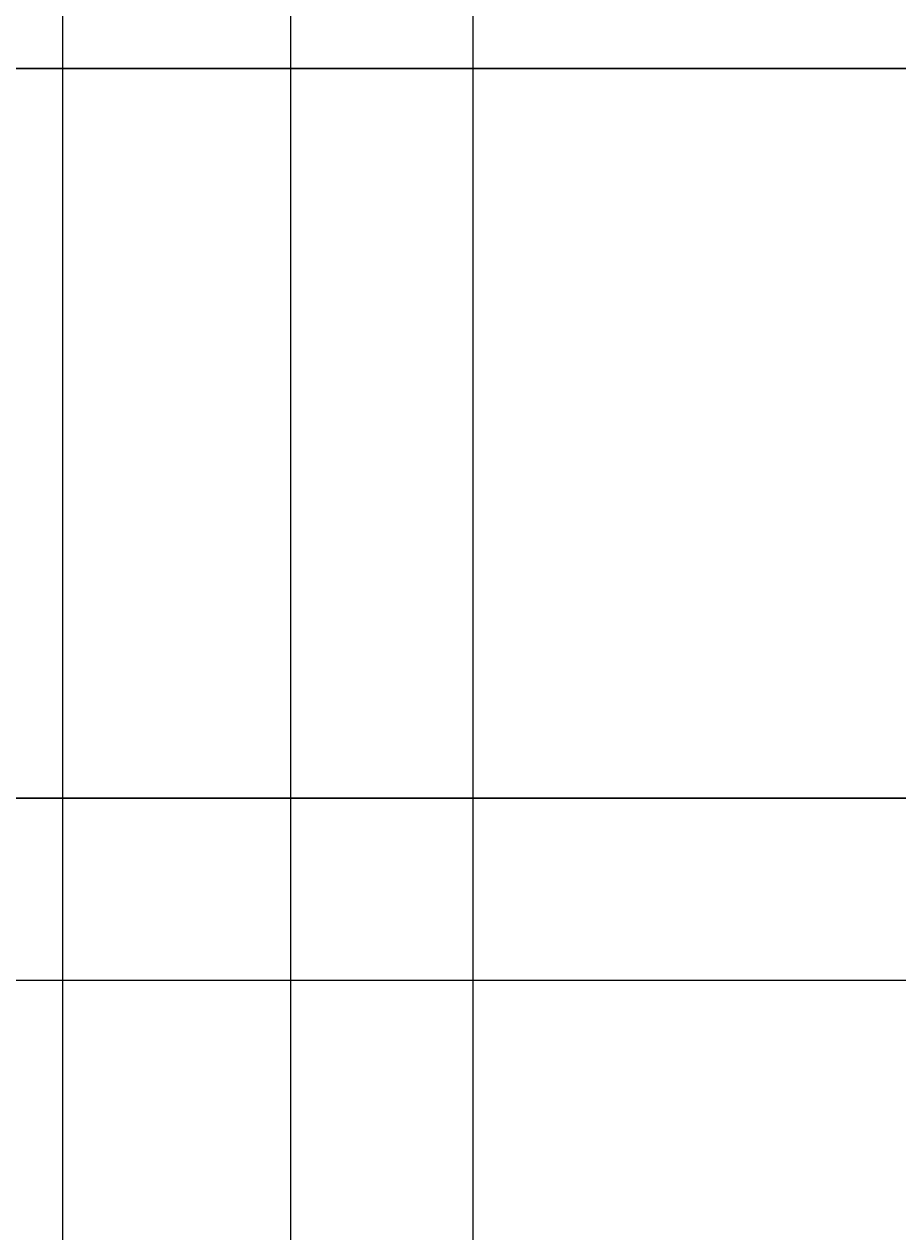
# Model space of a CAD drawing. Units: feet. Extents: x 105 to 1094, y -88 to 588.
# Tile 32 of 59: x 365 to 384, y 518 to 544. Entities that reach past the tile are written whole.
import ezdxf

# ---------------------------------------------------------------- set-up
doc = ezdxf.new("R2010")
doc.units = ezdxf.units.FT
doc.header["$MEASUREMENT"] = 0
doc.layers.add('A-ANNO-DIMS', color=2, linetype='Continuous', lineweight=18)
doc.layers.add('A-FLOR-PROJ', color=8, linetype='Continuous', lineweight=25)
doc.styles.get("Standard").update_dxf_attribs({"font": 'arial.ttf'})
doc.dimstyles.get("Standard").update_dxf_attribs({"dimtxt": 0.18, "dimasz": 0.18, "dimexe": 0.18, "dimexo": 0.0625, "dimgap": 0.09, "dimtad": 0, "dimtih": 1, "dimtoh": 1, "dimdec": 4, "dimzin": 0, "dimdsep": 46, "dimtxsty": 'Standard', "dimcen": 0.09, "dimadec": 0, "dimazin": 0, "dimtfac": 1, "dimtdec": 4, "dimtofl": 0, "dimtmove": 0, "dimatfit": 3, "dimfxl": 1, "dimtolj": 1, "dimtzin": 0, "dimarcsym": 0})

# ---------------------------------------------------------------- blocks, each defined once
blk = doc.blocks.new('*D21')
at = {"layer": 'A-ANNO-DIMS', "color": 0, "lineweight": -2, "transparency": 16777216}
for p, q in [((849.626, 543.081), (105.458, 543.081)), ((105.638, 542.901), (105.638, 250.263)), ((105.638, -42.739), (105.638, 249.899)), ((849.626, -42.919), (105.458, -42.919))]:
    blk.add_line(p, q, dxfattribs=at)
at = {"layer": 'A-ANNO-DIMS', "color": 0, "transparency": 16777216}
for points in [[(105.608, 542.901), (105.668, 542.901), (105.638, 543.081)], [(105.608, -42.739), (105.668, -42.739), (105.638, -42.919)]]:
    blk.add_solid(points, dxfattribs=at)
at = {"layer": 'Defpoints', "color": 0, "transparency": 16777216}
for p in [(105.638, 543.081), (849.688, 543.081), (849.688, -42.919)]:
    blk.add_point(p, dxfattribs=at)
at = {"layer": 'A-ANNO-DIMS', "color": 0, "transparency": 16777216, "insert": (105.638, 250.081), "char_height": 0.18, "attachment_point": 5}
blk.add_mtext('\\A1;586', dxfattribs=at)
blk = doc.blocks.new('*D24')
at = {"layer": 'A-ANNO-DIMS', "color": 0, "lineweight": -2, "transparency": 16777216}
for p, q in [((349.688, 543.144), (349.688, 588.311)), ((438.688, 527.144), (438.688, 588.311)), ((349.868, 588.131), (393.969, 588.131)), ((438.508, 588.131), (394.408, 588.131))]:
    blk.add_line(p, q, dxfattribs=at)
at = {"layer": 'A-ANNO-DIMS', "color": 0, "transparency": 16777216}
for points in [[(349.868, 588.161), (349.868, 588.101), (349.688, 588.131)], [(438.508, 588.161), (438.508, 588.101), (438.688, 588.131)]]:
    blk.add_solid(points, dxfattribs=at)
at = {"layer": 'Defpoints', "color": 0, "transparency": 16777216}
for p in [(438.688, 588.131), (349.688, 543.081), (438.688, 527.081)]:
    blk.add_point(p, dxfattribs=at)
at = {"layer": 'A-ANNO-DIMS', "color": 0, "transparency": 16777216, "insert": (394.188, 588.131), "char_height": 0.18, "attachment_point": 5}
blk.add_mtext('\\A1;89', dxfattribs=at)
blk = doc.blocks.new('*D30')
at = {"layer": 'A-ANNO-DIMS', "color": 0, "lineweight": -2, "transparency": 16777216}
for p, q in [((349.751, 543.081), (1093.918, 543.081)), ((1093.738, 542.901), (1093.738, 535.263)), ((1093.738, 527.261), (1093.738, 534.899)), ((349.751, 527.081), (1093.918, 527.081))]:
    blk.add_line(p, q, dxfattribs=at)
at = {"layer": 'A-ANNO-DIMS', "color": 0, "transparency": 16777216}
for points in [[(1093.708, 542.901), (1093.768, 542.901), (1093.738, 543.081)], [(1093.708, 527.261), (1093.768, 527.261), (1093.738, 527.081)]]:
    blk.add_solid(points, dxfattribs=at)
at = {"layer": 'Defpoints', "color": 0, "transparency": 16777216}
for p in [(349.688, 543.081), (349.688, 527.081), (1093.738, 527.081)]:
    blk.add_point(p, dxfattribs=at)
at = {"layer": 'A-ANNO-DIMS', "color": 0, "transparency": 16777216, "insert": (1093.738, 535.081), "char_height": 0.18, "attachment_point": 5}
blk.add_mtext('\\A1;16', dxfattribs=at)
blk = doc.blocks.new('*D39')
at = {"layer": 'A-ANNO-DIMS', "color": 0, "lineweight": -2, "transparency": 16777216}
for p, q in [((294.688, 204.144), (294.688, 588.311)), ((370.688, 204.144), (370.688, 588.311)), ((294.868, 588.131), (332.47, 588.131)), ((370.508, 588.131), (332.906, 588.131))]:
    blk.add_line(p, q, dxfattribs=at)
at = {"layer": 'A-ANNO-DIMS', "color": 0, "transparency": 16777216}
for points in [[(294.868, 588.161), (294.868, 588.101), (294.688, 588.131)], [(370.508, 588.161), (370.508, 588.101), (370.688, 588.131)]]:
    blk.add_solid(points, dxfattribs=at)
at = {"layer": 'Defpoints', "color": 0, "transparency": 16777216}
for p in [(370.688, 588.131), (294.688, 204.081), (370.688, 204.081)]:
    blk.add_point(p, dxfattribs=at)
at = {"layer": 'A-ANNO-DIMS', "color": 0, "transparency": 16777216, "insert": (332.688, 588.131), "char_height": 0.18, "attachment_point": 5}
blk.add_mtext('\\A1;76', dxfattribs=at)
blk = doc.blocks.new('*D53')
at = {"layer": 'A-ANNO-DIMS', "color": 0, "lineweight": -2, "transparency": 16777216}
for p, q in [((365.688, 394.144), (365.688, 588.311)), ((414.688, 394.144), (414.688, 588.311)), ((365.868, 588.131), (389.966, 588.131)), ((414.508, 588.131), (390.411, 588.131))]:
    blk.add_line(p, q, dxfattribs=at)
at = {"layer": 'A-ANNO-DIMS', "color": 0, "transparency": 16777216}
for points in [[(365.868, 588.161), (365.868, 588.101), (365.688, 588.131)], [(414.508, 588.161), (414.508, 588.101), (414.688, 588.131)]]:
    blk.add_solid(points, dxfattribs=at)
at = {"layer": 'Defpoints', "color": 0, "transparency": 16777216}
for p in [(365.688, 588.131), (365.688, 394.081), (414.688, 394.081)]:
    blk.add_point(p, dxfattribs=at)
at = {"layer": 'A-ANNO-DIMS', "color": 0, "transparency": 16777216, "insert": (390.188, 588.131), "char_height": 0.18, "attachment_point": 5}
blk.add_mtext('\\A1;49', dxfattribs=at)
blk = doc.blocks.new('*D56')
at = {"layer": 'A-ANNO-DIMS', "color": 0, "lineweight": -2, "transparency": 16777216}
for p, q in [((374.688, 252.144), (374.688, 588.311)), ((422.688, 252.144), (422.688, 588.311)), ((374.868, 588.131), (398.466, 588.131)), ((422.508, 588.131), (398.911, 588.131))]:
    blk.add_line(p, q, dxfattribs=at)
at = {"layer": 'A-ANNO-DIMS', "color": 0, "transparency": 16777216}
for points in [[(374.868, 588.161), (374.868, 588.101), (374.688, 588.131)], [(422.508, 588.161), (422.508, 588.101), (422.688, 588.131)]]:
    blk.add_solid(points, dxfattribs=at)
at = {"layer": 'Defpoints', "color": 0, "transparency": 16777216}
for p in [(422.688, 588.131), (374.688, 252.081), (422.688, 252.081)]:
    blk.add_point(p, dxfattribs=at)
at = {"layer": 'A-ANNO-DIMS', "color": 0, "transparency": 16777216, "insert": (398.688, 588.131), "char_height": 0.18, "attachment_point": 5}
blk.add_mtext('\\A1;48', dxfattribs=at)

msp = doc.modelspace()

# ---------------------------------------------------------------- linework, layer by layer
at = {"layer": 'A-FLOR-PROJ'}
for p, q in [((438.6883, 527.0812), (349.6883, 527.0812)), ((434.6883, 523.0812), (349.6883, 523.0812))]:
    msp.add_line(p, q, dxfattribs=at)

# ---------------------------------------------------------------- dimensions: what is measured, and where the dimension line sits
at = {"layer": 'A-ANNO-DIMS'}
for base, p1, p2, picture, middle in [((370.6883, 588.1312), (294.6883, 204.0812), (370.6883, 204.0812), '*D39', (332.6883, 588.1312)), ((438.6883, 588.1312), (349.6883, 543.0812), (438.6883, 527.0812), '*D24', (394.1883, 588.1312)), ((365.6883, 588.1312), (414.6883, 394.0812), (365.6883, 394.0812), '*D53', (390.1883, 588.1312)), ((422.6883, 588.1312), (374.6883, 252.0812), (422.6883, 252.0812), '*D56', (398.6883, 588.1312))]:
    dim = msp.add_linear_dim(base=base, p1=p1, p2=p2, dimstyle='Standard', override={"dimdec": 0, "dimlfac": 1, "dimrnd": 0, "dimzin": 0, "dimdsep": 46, "dimlunit": 2}, dxfattribs=at)
    dim.commit()
    dim.dimension.update_dxf_attribs({"geometry": picture, "text_midpoint": middle})
for base, p1, p2, picture, middle in [((105.6383, 543.0812), (849.6883, -42.9188), (849.6883, 543.0812), '*D21', (105.6383, 250.0812)), ((1093.7383, 527.0812), (349.6883, 543.0812), (349.6883, 527.0812), '*D30', (1093.7383, 535.0812))]:
    dim = msp.add_linear_dim(base=base, p1=p1, p2=p2, angle=90, dimstyle='Standard', override={"dimdec": 0, "dimlfac": 1, "dimrnd": 0, "dimzin": 0, "dimdsep": 46, "dimlunit": 2}, dxfattribs=at)
    dim.commit()
    dim.dimension.update_dxf_attribs({"geometry": picture, "text_midpoint": middle})

doc.saveas('drawing.dxf')
